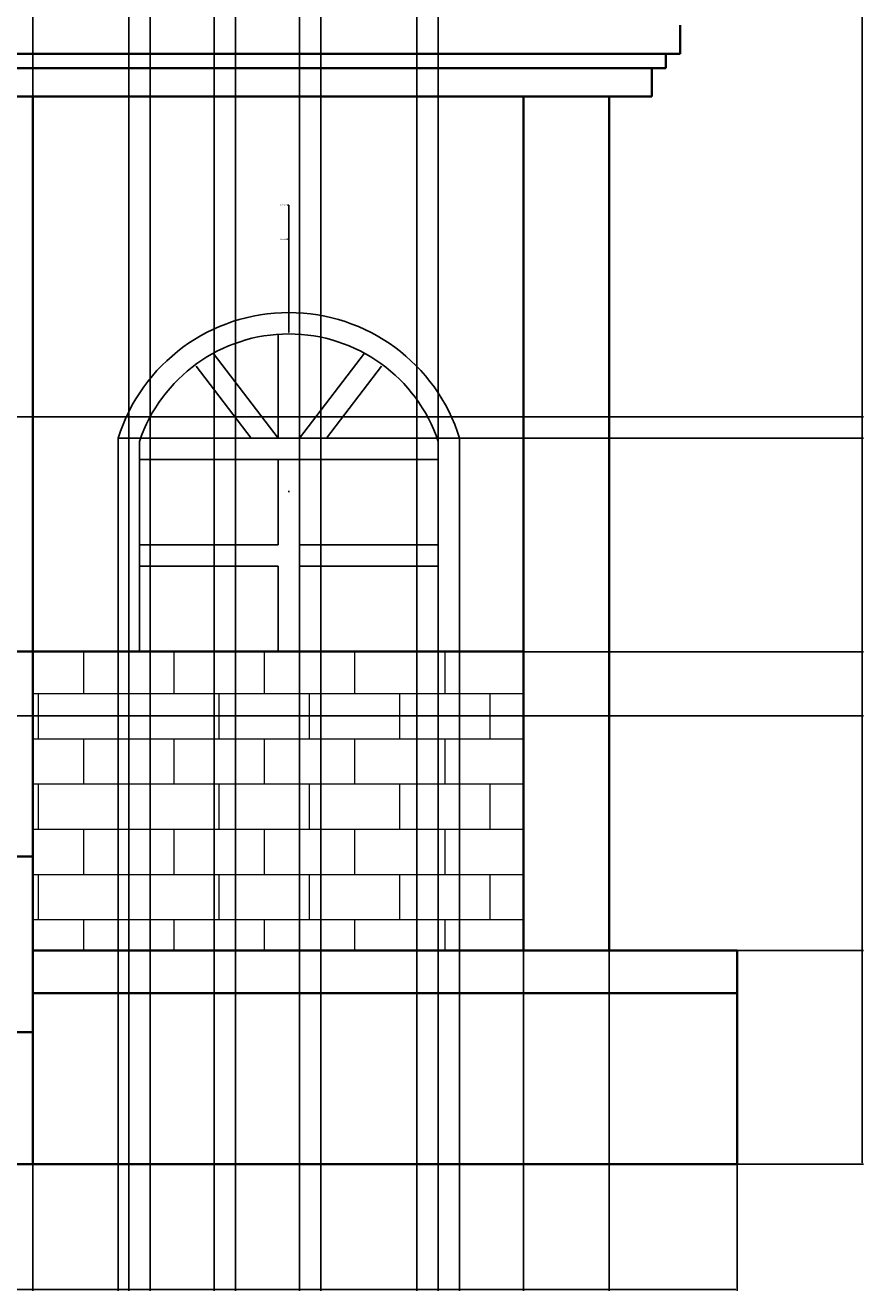
# Model space of a CAD drawing. Units: inches. Extents: x 2612 to 2948, y 481 to 865.
# Tile 4 of 7: x 2830 to 2948, y 481 to 659. Entities that reach past the tile are written whole.
import ezdxf

# ---------------------------------------------------------------- set-up
doc = ezdxf.new("R2010")
doc.units = ezdxf.units.IN
for name, color, linetype, lineweight in [('A-ANNO-DIMS', 2, 'Continuous', 18), ('A-COLS', 1, 'Continuous', 35), ('A-ELEV', 7, 'Continuous', 35), ('A-GLAZ', 4, 'Continuous', 25), ('A-WALL-PATT', 8, 'Continuous', 13)]:
    doc.layers.add(name, color=color, linetype=linetype, lineweight=lineweight)
doc.styles.get("Standard").update_dxf_attribs({"font": 'arial.ttf'})
doc.dimstyles.get("Standard").update_dxf_attribs({"dimtxt": 0.18, "dimasz": 0.18, "dimexe": 0.18, "dimexo": 0.0625, "dimgap": 0.09, "dimtad": 0, "dimtih": 1, "dimtoh": 1, "dimdec": 4, "dimzin": 0, "dimdsep": 46, "dimtxsty": 'Standard', "dimcen": 0.09, "dimadec": 0, "dimazin": 0, "dimtfac": 1, "dimtdec": 4, "dimtofl": 0, "dimtmove": 0, "dimatfit": 3, "dimfxl": 1, "dimtolj": 1, "dimtzin": 0, "dimarcsym": 0})

# ---------------------------------------------------------------- blocks, each defined once
blk = doc.blocks.new('*D12')
at = {"layer": 'A-ANNO-DIMS', "color": 0, "lineweight": -2, "transparency": 16777216}
for p, q in [((2930.37, 529.04), (2948.09, 529.04)), ((2947.91, 528.86), (2947.91, 514.23)), ((2947.91, 499.22), (2947.91, 513.86)), ((2930.37, 499.04), (2948.09, 499.04))]:
    blk.add_line(p, q, dxfattribs=at)
at = {"layer": 'A-ANNO-DIMS', "color": 0, "transparency": 16777216}
for points in [[(2947.88, 528.86), (2947.94, 528.86), (2947.91, 529.04)], [(2947.88, 499.22), (2947.94, 499.22), (2947.91, 499.04)]]:
    blk.add_solid(points, dxfattribs=at)
at = {"layer": 'Defpoints', "color": 0, "transparency": 16777216}
for p in [(2930.31, 529.04), (2947.91, 529.04), (2930.31, 499.04)]:
    blk.add_point(p, dxfattribs=at)
at = {"layer": 'A-ANNO-DIMS', "color": 0, "transparency": 16777216, "insert": (2947.91, 514.04), "char_height": 0.18, "attachment_point": 5}
blk.add_mtext('\\A1;30', dxfattribs=at)
blk = doc.blocks.new('*D13')
at = {"layer": 'A-ANNO-DIMS', "color": 0, "lineweight": -2, "transparency": 16777216}
for p, q in [((2843.37, 571.04), (2948.09, 571.04)), ((2947.91, 570.86), (2947.91, 550.22)), ((2947.91, 529.22), (2947.91, 549.86)), ((2930.37, 529.04), (2948.09, 529.04))]:
    blk.add_line(p, q, dxfattribs=at)
at = {"layer": 'A-ANNO-DIMS', "color": 0, "transparency": 16777216}
for points in [[(2947.88, 570.86), (2947.94, 570.86), (2947.91, 571.04)], [(2947.88, 529.22), (2947.94, 529.22), (2947.91, 529.04)]]:
    blk.add_solid(points, dxfattribs=at)
at = {"layer": 'Defpoints', "color": 0, "transparency": 16777216}
for p in [(2843.31, 571.04), (2947.91, 571.04), (2930.31, 529.04)]:
    blk.add_point(p, dxfattribs=at)
at = {"layer": 'A-ANNO-DIMS', "color": 0, "transparency": 16777216, "insert": (2947.91, 550.04), "char_height": 0.18, "attachment_point": 5}
blk.add_mtext('\\A1;42', dxfattribs=at)
blk = doc.blocks.new('*D14')
at = {"layer": 'A-ANNO-DIMS', "color": 0, "lineweight": -2, "transparency": 16777216}
for p, q in [((2843.37, 601.04), (2948.09, 601.04)), ((2947.91, 600.86), (2947.91, 586.23)), ((2947.91, 571.22), (2947.91, 585.86)), ((2843.37, 571.04), (2948.09, 571.04))]:
    blk.add_line(p, q, dxfattribs=at)
at = {"layer": 'A-ANNO-DIMS', "color": 0, "transparency": 16777216}
for points in [[(2947.88, 600.86), (2947.94, 600.86), (2947.91, 601.04)], [(2947.88, 571.22), (2947.94, 571.22), (2947.91, 571.04)]]:
    blk.add_solid(points, dxfattribs=at)
at = {"layer": 'Defpoints', "color": 0, "transparency": 16777216}
for p in [(2843.31, 601.04), (2947.91, 601.04), (2843.31, 571.04)]:
    blk.add_point(p, dxfattribs=at)
at = {"layer": 'A-ANNO-DIMS', "color": 0, "transparency": 16777216, "insert": (2947.91, 586.04), "char_height": 0.18, "attachment_point": 5}
blk.add_mtext('\\A1;30', dxfattribs=at)
blk = doc.blocks.new('*D22')
at = {"layer": 'A-ANNO-DIMS', "color": 0, "lineweight": -2, "transparency": 16777216}
for p, q in [((2708.31, 648.98), (2708.31, 481.26)), ((2831.31, 570.98), (2831.31, 481.26)), ((2708.49, 481.44), (2769.53, 481.44)), ((2831.13, 481.44), (2770.09, 481.44))]:
    blk.add_line(p, q, dxfattribs=at)
at = {"layer": 'A-ANNO-DIMS', "color": 0, "transparency": 16777216}
for points in [[(2708.49, 481.47), (2708.49, 481.41), (2708.31, 481.44)], [(2831.13, 481.47), (2831.13, 481.41), (2831.31, 481.44)]]:
    blk.add_solid(points, dxfattribs=at)
at = {"layer": 'Defpoints', "color": 0, "transparency": 16777216}
for p in [(2708.31, 649.04), (2831.31, 571.04), (2831.31, 481.44)]:
    blk.add_point(p, dxfattribs=at)
at = {"layer": 'A-ANNO-DIMS', "color": 0, "transparency": 16777216, "insert": (2769.81, 481.44), "char_height": 0.18, "attachment_point": 5}
blk.add_mtext('\\A1;123', dxfattribs=at)
blk = doc.blocks.new('*D23')
at = {"layer": 'A-ANNO-DIMS', "color": 0, "lineweight": -2, "transparency": 16777216}
for p, q in [((2831.31, 570.98), (2831.31, 481.26)), ((2843.31, 570.98), (2843.31, 481.26)), ((2831.49, 481.44), (2837.1, 481.44)), ((2843.13, 481.44), (2837.52, 481.44))]:
    blk.add_line(p, q, dxfattribs=at)
at = {"layer": 'A-ANNO-DIMS', "color": 0, "transparency": 16777216}
for points in [[(2831.49, 481.47), (2831.49, 481.41), (2831.31, 481.44)], [(2843.13, 481.47), (2843.13, 481.41), (2843.31, 481.44)]]:
    blk.add_solid(points, dxfattribs=at)
at = {"layer": 'Defpoints', "color": 0, "transparency": 16777216}
for p in [(2831.31, 571.04), (2843.31, 571.04), (2843.31, 481.44)]:
    blk.add_point(p, dxfattribs=at)
at = {"layer": 'A-ANNO-DIMS', "color": 0, "transparency": 16777216, "insert": (2837.31, 481.44), "char_height": 0.18, "attachment_point": 5}
blk.add_mtext('\\A1;12', dxfattribs=at)
blk = doc.blocks.new('*D24')
at = {"layer": 'A-ANNO-DIMS', "color": 0, "lineweight": -2, "transparency": 16777216}
for p, q in [((2843.31, 570.98), (2843.31, 481.26)), ((2891.31, 570.98), (2891.31, 481.26)), ((2843.49, 481.44), (2867.08, 481.44)), ((2891.13, 481.44), (2867.53, 481.44))]:
    blk.add_line(p, q, dxfattribs=at)
at = {"layer": 'A-ANNO-DIMS', "color": 0, "transparency": 16777216}
for points in [[(2843.49, 481.47), (2843.49, 481.41), (2843.31, 481.44)], [(2891.13, 481.47), (2891.13, 481.41), (2891.31, 481.44)]]:
    blk.add_solid(points, dxfattribs=at)
at = {"layer": 'Defpoints', "color": 0, "transparency": 16777216}
for p in [(2843.31, 571.04), (2891.31, 571.04), (2891.31, 481.44)]:
    blk.add_point(p, dxfattribs=at)
at = {"layer": 'A-ANNO-DIMS', "color": 0, "transparency": 16777216, "insert": (2867.31, 481.44), "char_height": 0.18, "attachment_point": 5}
blk.add_mtext('\\A1;48', dxfattribs=at)
blk = doc.blocks.new('*D25')
at = {"layer": 'A-ANNO-DIMS', "color": 0, "lineweight": -2, "transparency": 16777216}
for p, q in [((2891.31, 570.98), (2891.31, 481.26)), ((2900.31, 570.98), (2900.31, 481.26)), ((2891.49, 481.44), (2895.66, 481.44)), ((2900.13, 481.44), (2895.96, 481.44))]:
    blk.add_line(p, q, dxfattribs=at)
at = {"layer": 'A-ANNO-DIMS', "color": 0, "transparency": 16777216}
for points in [[(2891.49, 481.47), (2891.49, 481.41), (2891.31, 481.44)], [(2900.13, 481.47), (2900.13, 481.41), (2900.31, 481.44)]]:
    blk.add_solid(points, dxfattribs=at)
at = {"layer": 'Defpoints', "color": 0, "transparency": 16777216}
for p in [(2891.31, 571.04), (2900.31, 571.04), (2900.31, 481.44)]:
    blk.add_point(p, dxfattribs=at)
at = {"layer": 'A-ANNO-DIMS', "color": 0, "transparency": 16777216, "insert": (2895.81, 481.44), "char_height": 0.18, "attachment_point": 5}
blk.add_mtext('\\A1;9', dxfattribs=at)
blk = doc.blocks.new('*D26')
at = {"layer": 'A-ANNO-DIMS', "color": 0, "lineweight": -2, "transparency": 16777216}
for p, q in [((2900.31, 528.98), (2900.31, 481.26)), ((2912.31, 528.98), (2912.31, 481.26)), ((2900.49, 481.44), (2906.1, 481.44)), ((2912.13, 481.44), (2906.52, 481.44))]:
    blk.add_line(p, q, dxfattribs=at)
at = {"layer": 'A-ANNO-DIMS', "color": 0, "transparency": 16777216}
for points in [[(2900.49, 481.47), (2900.49, 481.41), (2900.31, 481.44)], [(2912.13, 481.47), (2912.13, 481.41), (2912.31, 481.44)]]:
    blk.add_solid(points, dxfattribs=at)
at = {"layer": 'Defpoints', "color": 0, "transparency": 16777216}
for p in [(2900.31, 529.04), (2912.31, 529.04), (2912.31, 481.44)]:
    blk.add_point(p, dxfattribs=at)
at = {"layer": 'A-ANNO-DIMS', "color": 0, "transparency": 16777216, "insert": (2906.31, 481.44), "char_height": 0.18, "attachment_point": 5}
blk.add_mtext('\\A1;12', dxfattribs=at)
blk = doc.blocks.new('*D27')
at = {"layer": 'A-ANNO-DIMS', "color": 0, "lineweight": -2, "transparency": 16777216}
for p, q in [((2912.31, 528.98), (2912.31, 481.26)), ((2930.31, 528.98), (2930.31, 481.26)), ((2912.49, 481.44), (2921.1, 481.44)), ((2930.13, 481.44), (2921.52, 481.44))]:
    blk.add_line(p, q, dxfattribs=at)
at = {"layer": 'A-ANNO-DIMS', "color": 0, "transparency": 16777216}
for points in [[(2912.49, 481.47), (2912.49, 481.41), (2912.31, 481.44)], [(2930.13, 481.47), (2930.13, 481.41), (2930.31, 481.44)]]:
    blk.add_solid(points, dxfattribs=at)
at = {"layer": 'Defpoints', "color": 0, "transparency": 16777216}
for p in [(2912.31, 529.04), (2930.31, 529.04), (2930.31, 481.44)]:
    blk.add_point(p, dxfattribs=at)
at = {"layer": 'A-ANNO-DIMS', "color": 0, "transparency": 16777216, "insert": (2921.31, 481.44), "char_height": 0.18, "attachment_point": 5}
blk.add_mtext('\\A1;18', dxfattribs=at)
blk = doc.blocks.new('*D64')
at = {"layer": 'A-ANNO-DIMS', "color": 0, "lineweight": -2, "transparency": 16777216}
for p, q in [((2826.87, 562.04), (2948.09, 562.04)), ((2947.91, 561.86), (2947.91, 530.73)), ((2947.91, 499.22), (2947.91, 530.36)), ((2826.87, 499.04), (2948.09, 499.04))]:
    blk.add_line(p, q, dxfattribs=at)
at = {"layer": 'A-ANNO-DIMS', "color": 0, "transparency": 16777216}
for points in [[(2947.88, 561.86), (2947.94, 561.86), (2947.91, 562.04)], [(2947.88, 499.22), (2947.94, 499.22), (2947.91, 499.04)]]:
    blk.add_solid(points, dxfattribs=at)
at = {"layer": 'Defpoints', "color": 0, "transparency": 16777216}
for p in [(2826.81, 562.04), (2947.91, 562.04), (2826.81, 499.04)]:
    blk.add_point(p, dxfattribs=at)
at = {"layer": 'A-ANNO-DIMS', "color": 0, "transparency": 16777216, "insert": (2947.91, 530.54), "char_height": 0.18, "attachment_point": 5}
blk.add_mtext('\\A1;63', dxfattribs=at)
blk = doc.blocks.new('*D65')
at = {"layer": 'A-ANNO-DIMS', "color": 0, "lineweight": -2, "transparency": 16777216}
for p, q in [((2793.87, 604.04), (2948.09, 604.04)), ((2947.91, 603.86), (2947.91, 583.22)), ((2947.91, 562.22), (2947.91, 582.86)), ((2793.87, 562.04), (2948.09, 562.04))]:
    blk.add_line(p, q, dxfattribs=at)
at = {"layer": 'A-ANNO-DIMS', "color": 0, "transparency": 16777216}
for points in [[(2947.88, 603.86), (2947.94, 603.86), (2947.91, 604.04)], [(2947.88, 562.22), (2947.94, 562.22), (2947.91, 562.04)]]:
    blk.add_solid(points, dxfattribs=at)
at = {"layer": 'Defpoints', "color": 0, "transparency": 16777216}
for p in [(2793.81, 604.04), (2947.91, 604.04), (2793.81, 562.04)]:
    blk.add_point(p, dxfattribs=at)
at = {"layer": 'A-ANNO-DIMS', "color": 0, "transparency": 16777216, "insert": (2947.91, 583.04), "char_height": 0.18, "attachment_point": 5}
blk.add_mtext('\\A1;42', dxfattribs=at)
blk = doc.blocks.new('*D74')
at = {"layer": 'A-ANNO-DIMS', "color": 0, "lineweight": -2, "transparency": 16777216}
for p, q in [((2831.31, 711.98), (2831.31, 481.26)), ((2828.31, 708.98), (2828.31, 481.26)), ((2828.49, 481.44), (2829.66, 481.44)), ((2831.13, 481.44), (2829.96, 481.44))]:
    blk.add_line(p, q, dxfattribs=at)
at = {"layer": 'A-ANNO-DIMS', "color": 0, "transparency": 16777216}
for points in [[(2828.49, 481.47), (2828.49, 481.41), (2828.31, 481.44)], [(2831.13, 481.47), (2831.13, 481.41), (2831.31, 481.44)]]:
    blk.add_solid(points, dxfattribs=at)
at = {"layer": 'Defpoints', "color": 0, "transparency": 16777216}
for p in [(2831.31, 712.04), (2828.31, 709.04), (2831.31, 481.44)]:
    blk.add_point(p, dxfattribs=at)
at = {"layer": 'A-ANNO-DIMS', "color": 0, "transparency": 16777216, "insert": (2829.81, 481.44), "char_height": 0.18, "attachment_point": 5}
blk.add_mtext('\\A1;3', dxfattribs=at)
blk = doc.blocks.new('*D75')
at = {"layer": 'A-ANNO-DIMS', "color": 0, "lineweight": -2, "transparency": 16777216}
for p, q in [((2831.31, 711.98), (2831.31, 481.26)), ((2844.81, 711.98), (2844.81, 481.26)), ((2831.49, 481.44), (2837.74, 481.44)), ((2844.63, 481.44), (2838.37, 481.44))]:
    blk.add_line(p, q, dxfattribs=at)
at = {"layer": 'A-ANNO-DIMS', "color": 0, "transparency": 16777216}
for points in [[(2831.49, 481.47), (2831.49, 481.41), (2831.31, 481.44)], [(2844.63, 481.47), (2844.63, 481.41), (2844.81, 481.44)]]:
    blk.add_solid(points, dxfattribs=at)
at = {"layer": 'Defpoints', "color": 0, "transparency": 16777216}
for p in [(2831.31, 712.04), (2844.81, 712.04), (2844.81, 481.44)]:
    blk.add_point(p, dxfattribs=at)
at = {"layer": 'A-ANNO-DIMS', "color": 0, "transparency": 16777216, "insert": (2838.06, 481.44), "char_height": 0.18, "attachment_point": 5}
blk.add_mtext('\\A1;13.5', dxfattribs=at)
blk = doc.blocks.new('*D76')
at = {"layer": 'A-ANNO-DIMS', "color": 0, "lineweight": -2, "transparency": 16777216}
for p, q in [((2844.81, 711.98), (2844.81, 481.26)), ((2847.81, 711.98), (2847.81, 481.26)), ((2844.99, 481.44), (2846.16, 481.44)), ((2847.63, 481.44), (2846.46, 481.44))]:
    blk.add_line(p, q, dxfattribs=at)
at = {"layer": 'A-ANNO-DIMS', "color": 0, "transparency": 16777216}
for points in [[(2844.99, 481.47), (2844.99, 481.41), (2844.81, 481.44)], [(2847.63, 481.47), (2847.63, 481.41), (2847.81, 481.44)]]:
    blk.add_solid(points, dxfattribs=at)
at = {"layer": 'Defpoints', "color": 0, "transparency": 16777216}
for p in [(2844.81, 712.04), (2847.81, 712.04), (2847.81, 481.44)]:
    blk.add_point(p, dxfattribs=at)
at = {"layer": 'A-ANNO-DIMS', "color": 0, "transparency": 16777216, "insert": (2846.31, 481.44), "char_height": 0.18, "attachment_point": 5}
blk.add_mtext('\\A1;3', dxfattribs=at)
blk = doc.blocks.new('*D77')
at = {"layer": 'A-ANNO-DIMS', "color": 0, "lineweight": -2, "transparency": 16777216}
for p, q in [((2847.81, 711.98), (2847.81, 481.26)), ((2856.81, 711.98), (2856.81, 481.26)), ((2847.99, 481.44), (2852.16, 481.44)), ((2856.63, 481.44), (2852.46, 481.44))]:
    blk.add_line(p, q, dxfattribs=at)
at = {"layer": 'A-ANNO-DIMS', "color": 0, "transparency": 16777216}
for points in [[(2847.99, 481.47), (2847.99, 481.41), (2847.81, 481.44)], [(2856.63, 481.47), (2856.63, 481.41), (2856.81, 481.44)]]:
    blk.add_solid(points, dxfattribs=at)
at = {"layer": 'Defpoints', "color": 0, "transparency": 16777216}
for p in [(2847.81, 712.04), (2856.81, 712.04), (2856.81, 481.44)]:
    blk.add_point(p, dxfattribs=at)
at = {"layer": 'A-ANNO-DIMS', "color": 0, "transparency": 16777216, "insert": (2852.31, 481.44), "char_height": 0.18, "attachment_point": 5}
blk.add_mtext('\\A1;9', dxfattribs=at)
blk = doc.blocks.new('*D78')
at = {"layer": 'A-ANNO-DIMS', "color": 0, "lineweight": -2, "transparency": 16777216}
for p, q in [((2856.81, 711.98), (2856.81, 481.26)), ((2859.81, 711.98), (2859.81, 481.26)), ((2856.99, 481.44), (2858.16, 481.44)), ((2859.63, 481.44), (2858.46, 481.44))]:
    blk.add_line(p, q, dxfattribs=at)
at = {"layer": 'A-ANNO-DIMS', "color": 0, "transparency": 16777216}
for points in [[(2856.99, 481.47), (2856.99, 481.41), (2856.81, 481.44)], [(2859.63, 481.47), (2859.63, 481.41), (2859.81, 481.44)]]:
    blk.add_solid(points, dxfattribs=at)
at = {"layer": 'Defpoints', "color": 0, "transparency": 16777216}
for p in [(2856.81, 712.04), (2859.81, 712.04), (2859.81, 481.44)]:
    blk.add_point(p, dxfattribs=at)
at = {"layer": 'A-ANNO-DIMS', "color": 0, "transparency": 16777216, "insert": (2858.31, 481.44), "char_height": 0.18, "attachment_point": 5}
blk.add_mtext('\\A1;3', dxfattribs=at)
blk = doc.blocks.new('*D79')
at = {"layer": 'A-ANNO-DIMS', "color": 0, "lineweight": -2, "transparency": 16777216}
for p, q in [((2859.81, 711.98), (2859.81, 481.26)), ((2868.81, 711.98), (2868.81, 481.26)), ((2859.99, 481.44), (2864.16, 481.44)), ((2868.63, 481.44), (2864.46, 481.44))]:
    blk.add_line(p, q, dxfattribs=at)
at = {"layer": 'A-ANNO-DIMS', "color": 0, "transparency": 16777216}
for points in [[(2859.99, 481.47), (2859.99, 481.41), (2859.81, 481.44)], [(2868.63, 481.47), (2868.63, 481.41), (2868.81, 481.44)]]:
    blk.add_solid(points, dxfattribs=at)
at = {"layer": 'Defpoints', "color": 0, "transparency": 16777216}
for p in [(2859.81, 712.04), (2868.81, 712.04), (2868.81, 481.44)]:
    blk.add_point(p, dxfattribs=at)
at = {"layer": 'A-ANNO-DIMS', "color": 0, "transparency": 16777216, "insert": (2864.31, 481.44), "char_height": 0.18, "attachment_point": 5}
blk.add_mtext('\\A1;9', dxfattribs=at)
blk = doc.blocks.new('*D80')
at = {"layer": 'A-ANNO-DIMS', "color": 0, "lineweight": -2, "transparency": 16777216}
for p, q in [((2868.81, 711.98), (2868.81, 481.26)), ((2871.81, 711.98), (2871.81, 481.26)), ((2868.99, 481.44), (2870.16, 481.44)), ((2871.63, 481.44), (2870.46, 481.44))]:
    blk.add_line(p, q, dxfattribs=at)
at = {"layer": 'A-ANNO-DIMS', "color": 0, "transparency": 16777216}
for points in [[(2868.99, 481.47), (2868.99, 481.41), (2868.81, 481.44)], [(2871.63, 481.47), (2871.63, 481.41), (2871.81, 481.44)]]:
    blk.add_solid(points, dxfattribs=at)
at = {"layer": 'Defpoints', "color": 0, "transparency": 16777216}
for p in [(2868.81, 712.04), (2871.81, 712.04), (2871.81, 481.44)]:
    blk.add_point(p, dxfattribs=at)
at = {"layer": 'A-ANNO-DIMS', "color": 0, "transparency": 16777216, "insert": (2870.31, 481.44), "char_height": 0.18, "attachment_point": 5}
blk.add_mtext('\\A1;3', dxfattribs=at)
blk = doc.blocks.new('*D81')
at = {"layer": 'A-ANNO-DIMS', "color": 0, "lineweight": -2, "transparency": 16777216}
for p, q in [((2871.81, 711.98), (2871.81, 481.26)), ((2885.31, 711.98), (2885.31, 481.26)), ((2871.99, 481.44), (2878.24, 481.44)), ((2885.13, 481.44), (2878.87, 481.44))]:
    blk.add_line(p, q, dxfattribs=at)
at = {"layer": 'A-ANNO-DIMS', "color": 0, "transparency": 16777216}
for points in [[(2871.99, 481.47), (2871.99, 481.41), (2871.81, 481.44)], [(2885.13, 481.47), (2885.13, 481.41), (2885.31, 481.44)]]:
    blk.add_solid(points, dxfattribs=at)
at = {"layer": 'Defpoints', "color": 0, "transparency": 16777216}
for p in [(2871.81, 712.04), (2885.31, 712.04), (2885.31, 481.44)]:
    blk.add_point(p, dxfattribs=at)
at = {"layer": 'A-ANNO-DIMS', "color": 0, "transparency": 16777216, "insert": (2878.56, 481.44), "char_height": 0.18, "attachment_point": 5}
blk.add_mtext('\\A1;13.5', dxfattribs=at)
blk = doc.blocks.new('*D82')
at = {"layer": 'A-ANNO-DIMS', "color": 0, "lineweight": -2, "transparency": 16777216}
for p, q in [((2885.31, 711.98), (2885.31, 481.26)), ((2888.31, 708.98), (2888.31, 481.26)), ((2885.49, 481.44), (2886.66, 481.44)), ((2888.13, 481.44), (2886.96, 481.44))]:
    blk.add_line(p, q, dxfattribs=at)
at = {"layer": 'A-ANNO-DIMS', "color": 0, "transparency": 16777216}
for points in [[(2885.49, 481.47), (2885.49, 481.41), (2885.31, 481.44)], [(2888.13, 481.47), (2888.13, 481.41), (2888.31, 481.44)]]:
    blk.add_solid(points, dxfattribs=at)
at = {"layer": 'Defpoints', "color": 0, "transparency": 16777216}
for p in [(2885.31, 712.04), (2888.31, 709.04), (2888.31, 481.44)]:
    blk.add_point(p, dxfattribs=at)
at = {"layer": 'A-ANNO-DIMS', "color": 0, "transparency": 16777216, "insert": (2886.81, 481.44), "char_height": 0.18, "attachment_point": 5}
blk.add_mtext('\\A1;3', dxfattribs=at)
blk = doc.blocks.new('*D86')
at = {"layer": 'A-ANNO-DIMS', "color": 0, "lineweight": -2, "transparency": 16777216}
for p, q in [((2930.37, 847.04), (2948.09, 847.04)), ((2947.91, 846.86), (2947.91, 673.23)), ((2947.91, 499.22), (2947.91, 672.86)), ((2930.37, 499.04), (2948.09, 499.04))]:
    blk.add_line(p, q, dxfattribs=at)
at = {"layer": 'A-ANNO-DIMS', "color": 0, "transparency": 16777216}
for points in [[(2947.88, 846.86), (2947.94, 846.86), (2947.91, 847.04)], [(2947.88, 499.22), (2947.94, 499.22), (2947.91, 499.04)]]:
    blk.add_solid(points, dxfattribs=at)
at = {"layer": 'Defpoints', "color": 0, "transparency": 16777216}
for p in [(2930.31, 847.04), (2947.91, 847.04), (2930.31, 499.04)]:
    blk.add_point(p, dxfattribs=at)
at = {"layer": 'A-ANNO-DIMS', "color": 0, "transparency": 16777216, "insert": (2947.91, 673.04), "char_height": 0.18, "attachment_point": 5}
blk.add_mtext('\\A1;348', dxfattribs=at)
blk = doc.blocks.new('*D87')
at = {"layer": 'A-ANNO-DIMS', "color": 0, "lineweight": -2, "transparency": 16777216}
for p, q in [((2630.31, 498.98), (2630.31, 481.26)), ((2930.31, 498.98), (2930.31, 481.26)), ((2630.49, 481.44), (2780.02, 481.44)), ((2930.13, 481.44), (2780.6, 481.44))]:
    blk.add_line(p, q, dxfattribs=at)
at = {"layer": 'A-ANNO-DIMS', "color": 0, "transparency": 16777216}
for points in [[(2630.49, 481.47), (2630.49, 481.41), (2630.31, 481.44)], [(2930.13, 481.47), (2930.13, 481.41), (2930.31, 481.44)]]:
    blk.add_solid(points, dxfattribs=at)
at = {"layer": 'Defpoints', "color": 0, "transparency": 16777216}
for p in [(2630.31, 499.04), (2930.31, 499.04), (2930.31, 481.44)]:
    blk.add_point(p, dxfattribs=at)
at = {"layer": 'A-ANNO-DIMS', "color": 0, "transparency": 16777216, "insert": (2780.31, 481.44), "char_height": 0.18, "attachment_point": 5}
blk.add_mtext('\\A1;300', dxfattribs=at)
blk = doc.blocks.new('*D88')
at = {"layer": 'A-ANNO-DIMS', "color": 0, "lineweight": -2, "transparency": 16777216}
for p, q in [((2867.13, 633.78), (2867.31, 633.78)), ((2867.31, 633.78), (2867.31, 618.87)), ((2867.22, 593.54), (2867.4, 593.54)), ((2867.31, 593.45), (2867.31, 593.63))]:
    blk.add_line(p, q, dxfattribs=at)
at = {"layer": 'A-ANNO-DIMS', "color": 0, "transparency": 16777216}
blk.add_solid([(2867.34, 618.87), (2867.28, 618.87), (2867.31, 618.69)], dxfattribs=at)
at = {"layer": 'Defpoints', "color": 0, "transparency": 16777216}
for p in [(2867.31, 618.69), (2867.31, 593.54)]:
    blk.add_point(p, dxfattribs=at)
at = {"layer": 'A-ANNO-DIMS', "color": 0, "transparency": 16777216, "insert": (2866.58, 633.78), "char_height": 0.18, "attachment_point": 5}
blk.add_mtext('\\A1;R25.145', dxfattribs=at)
blk = doc.blocks.new('*D89')
at = {"layer": 'A-ANNO-DIMS', "color": 0, "lineweight": -2, "transparency": 16777216}
for p, q in [((2867.13, 628.98), (2867.31, 628.98)), ((2867.31, 628.98), (2867.31, 615.87)), ((2867.22, 593.54), (2867.4, 593.54)), ((2867.31, 593.45), (2867.31, 593.63))]:
    blk.add_line(p, q, dxfattribs=at)
at = {"layer": 'A-ANNO-DIMS', "color": 0, "transparency": 16777216}
blk.add_solid([(2867.34, 615.87), (2867.28, 615.87), (2867.31, 615.69)], dxfattribs=at)
at = {"layer": 'Defpoints', "color": 0, "transparency": 16777216}
for p in [(2867.31, 615.69), (2867.31, 593.54)]:
    blk.add_point(p, dxfattribs=at)
at = {"layer": 'A-ANNO-DIMS', "color": 0, "transparency": 16777216, "insert": (2866.58, 628.98), "char_height": 0.18, "attachment_point": 5}
blk.add_mtext('\\A1;R22.145', dxfattribs=at)

msp = doc.modelspace()

# ---------------------------------------------------------------- hatches: boundary and pattern name
at = {"layer": 'A-WALL-PATT'}
h = msp.add_hatch(dxfattribs=at)
h.set_pattern_fill('BRICK', color=256)
h.paths.add_polyline_path([(2900.3074, 571.0443), (2831.3074, 571.0443), (2831.3074, 529.0443), (2900.3074, 529.0443)])

# ---------------------------------------------------------------- linework, layer by layer
at = {"layer": 'A-COLS'}
msp.add_line((2900.3074, 529.0443), (2900.3074, 649.0443), dxfattribs=at)
at = {"layer": 'A-ELEV'}
for p, q in [((2922.3074, 655.0443), (2922.3074, 659.0443)), ((2642.3074, 655.0443), (2918.3074, 655.0443)), ((2918.3074, 655.0443), (2920.3074, 655.0443)), ((2920.3074, 655.0443), (2922.3074, 655.0443)), ((2920.3074, 653.0443), (2920.3074, 655.0443)), ((2642.3074, 653.0443), (2918.3074, 653.0443)), ((2918.3074, 649.0443), (2918.3074, 653.0443)), ((2918.3074, 653.0443), (2920.3074, 653.0443)), ((2642.3074, 649.0443), (2918.3074, 649.0443)), ((2831.3074, 499.0443), (2831.3074, 649.0443)), ((2912.3074, 529.0443), (2912.3074, 649.0443)), ((2816.9214, 571.0443), (2900.3074, 571.0443)), ((2831.3074, 571.0443), (2816.9214, 571.0443)), ((2826.8074, 542.2613), (2831.3074, 542.2613)), ((2831.3074, 529.0443), (2900.3074, 529.0443)), ((2900.3074, 529.0443), (2930.3074, 529.0443)), ((2930.3074, 499.0443), (2930.3074, 529.0443)), ((2831.3074, 523.0443), (2900.3074, 523.0443)), ((2900.3074, 523.0443), (2930.3074, 523.0443)), ((2826.8074, 517.5686), (2831.3074, 517.5686)), ((2630.3074, 499.0443), (2930.3074, 499.0443))]:
    msp.add_line(p, q, dxfattribs=at)
at = {"layer": 'A-GLAZ'}
for p, q in [((2865.8074, 601.0443), (2865.8074, 615.6889)), ((2868.8074, 601.0443), (2868.8074, 615.6889)), ((2865.8074, 601.0443), (2856.6574, 612.9597)), ((2868.8074, 601.0443), (2877.9575, 612.9597)), ((2862.0249, 601.0443), (2854.278, 611.1326)), ((2872.5899, 601.0443), (2880.3368, 611.1326)), ((2843.3074, 571.0443), (2843.3074, 601.0443)), ((2846.4716, 601.0443), (2862.0249, 601.0443)), ((2872.5899, 601.0443), (2888.1433, 601.0443)), ((2891.3074, 571.0443), (2891.3074, 601.0443)), ((2846.3074, 571.0443), (2846.3074, 600.5715)), ((2888.3074, 571.0443), (2888.3074, 600.5715)), ((2846.3074, 598.0443), (2865.8074, 598.0443)), ((2865.8074, 598.0443), (2865.8074, 586.0443)), ((2865.8074, 598.0443), (2888.3074, 598.0443)), ((2868.8074, 598.0443), (2868.8074, 586.0443)), ((2846.3074, 586.0443), (2865.8074, 586.0443)), ((2868.8074, 586.0443), (2888.3074, 586.0443)), ((2846.3074, 583.0443), (2865.8074, 583.0443)), ((2865.8074, 583.0443), (2865.8074, 571.0443)), ((2865.8074, 583.0443), (2865.8074, 571.0443)), ((2868.8074, 583.0443), (2868.8074, 571.0443)), ((2868.8074, 583.0443), (2888.3074, 583.0443)), ((2868.8074, 583.0443), (2868.8074, 571.0443)), ((2843.3074, 571.0443), (2891.3074, 571.0443))]:
    msp.add_line(p, q, dxfattribs=at)
for radius, start, end in [(25.1446, 17.354025, 162.645975), (22.1446, 18.501882, 161.498118)]:
    msp.add_arc((2867.3074, 593.5443), radius, start, end, dxfattribs=at)

# ---------------------------------------------------------------- dimensions: what is measured, and where the dimension line sits
at = {"layer": 'A-ANNO-DIMS'}
for base, p1, p2, picture, middle in [((2947.9074, 847.0443), (2930.3074, 499.0443), (2930.3074, 847.0443), '*D86', (2947.9074, 673.0443)), ((2947.9074, 604.0443), (2793.8074, 562.0443), (2793.8074, 604.0443), '*D65', (2947.9074, 583.0443)), ((2947.9074, 601.0443), (2843.3074, 571.0443), (2843.3074, 601.0443), '*D14', (2947.9074, 586.0443)), ((2947.9074, 571.0443), (2930.3074, 529.0443), (2843.3074, 571.0443), '*D13', (2947.9074, 550.0443)), ((2947.9074, 562.0443), (2826.8074, 499.0443), (2826.8074, 562.0443), '*D64', (2947.9074, 530.5443)), ((2947.9074, 529.0443), (2930.3074, 499.0443), (2930.3074, 529.0443), '*D12', (2947.9074, 514.0443))]:
    dim = msp.add_linear_dim(base=base, p1=p1, p2=p2, angle=90, dimstyle='Standard', override={"dimdec": 0, "dimlfac": 1, "dimrnd": 0, "dimzin": 0, "dimdsep": 46, "dimlunit": 2}, dxfattribs=at)
    dim.commit()
    dim.dimension.update_dxf_attribs({"geometry": picture, "text_midpoint": middle})
for base, p1, p2, override, picture, middle in [((2831.3074, 481.4443), (2828.3074, 709.0443), (2831.3074, 712.0443), {"dimdec": 0, "dimlfac": 1, "dimrnd": 0, "dimzin": 0, "dimdsep": 46, "dimlunit": 2}, '*D74', (2829.8074, 481.4443)), ((2844.8074, 481.4443), (2831.3074, 712.0443), (2844.8074, 712.0443), {"dimdec": 1, "dimlfac": 1, "dimrnd": 0, "dimzin": 0, "dimdsep": 46, "dimlunit": 2}, '*D75', (2838.0574, 481.4443)), ((2847.8074, 481.4443), (2844.8074, 712.0443), (2847.8074, 712.0443), {"dimdec": 0, "dimlfac": 1, "dimrnd": 0, "dimzin": 0, "dimdsep": 46, "dimlunit": 2}, '*D76', (2846.3074, 481.4443)), ((2856.8074, 481.4443), (2847.8074, 712.0443), (2856.8074, 712.0443), {"dimdec": 0, "dimlfac": 1, "dimrnd": 0, "dimzin": 0, "dimdsep": 46, "dimlunit": 2}, '*D77', (2852.3074, 481.4443)), ((2859.8074, 481.4443), (2856.8074, 712.0443), (2859.8074, 712.0443), {"dimdec": 0, "dimlfac": 1, "dimrnd": 0, "dimzin": 0, "dimdsep": 46, "dimlunit": 2}, '*D78', (2858.3074, 481.4443)), ((2868.8074, 481.4443), (2859.8074, 712.0443), (2868.8074, 712.0443), {"dimdec": 0, "dimlfac": 1, "dimrnd": 0, "dimzin": 0, "dimdsep": 46, "dimlunit": 2}, '*D79', (2864.3074, 481.4443)), ((2871.8074, 481.4443), (2868.8074, 712.0443), (2871.8074, 712.0443), {"dimdec": 0, "dimlfac": 1, "dimrnd": 0, "dimzin": 0, "dimdsep": 46, "dimlunit": 2}, '*D80', (2870.3074, 481.4443)), ((2885.3074, 481.4443), (2871.8074, 712.0443), (2885.3074, 712.0443), {"dimdec": 1, "dimlfac": 1, "dimrnd": 0, "dimzin": 0, "dimdsep": 46, "dimlunit": 2}, '*D81', (2878.5574, 481.4443)), ((2888.3074, 481.4443), (2885.3074, 712.0443), (2888.3074, 709.0443), {"dimdec": 0, "dimlfac": 1, "dimrnd": 0, "dimzin": 0, "dimdsep": 46, "dimlunit": 2}, '*D82', (2886.8074, 481.4443)), ((2831.3074, 481.4443), (2708.3074, 649.0443), (2831.3074, 571.0443), {"dimdec": 0, "dimlfac": 1, "dimrnd": 0, "dimzin": 0, "dimdsep": 46, "dimlunit": 2}, '*D22', (2769.8074, 481.4443)), ((2843.3074, 481.4443), (2831.3074, 571.0443), (2843.3074, 571.0443), {"dimdec": 0, "dimlfac": 1, "dimrnd": 0, "dimzin": 0, "dimdsep": 46, "dimlunit": 2}, '*D23', (2837.3074, 481.4443)), ((2891.3074, 481.4443), (2843.3074, 571.0443), (2891.3074, 571.0443), {"dimdec": 0, "dimlfac": 1, "dimrnd": 0, "dimzin": 0, "dimdsep": 46, "dimlunit": 2}, '*D24', (2867.3074, 481.4443)), ((2900.3074, 481.4443), (2891.3074, 571.0443), (2900.3074, 571.0443), {"dimdec": 0, "dimlfac": 1, "dimrnd": 0, "dimzin": 0, "dimdsep": 46, "dimlunit": 2}, '*D25', (2895.8074, 481.4443)), ((2912.3074, 481.4443), (2900.3074, 529.0443), (2912.3074, 529.0443), {"dimdec": 0, "dimlfac": 1, "dimrnd": 0, "dimzin": 0, "dimdsep": 46, "dimlunit": 2}, '*D26', (2906.3074, 481.4443)), ((2930.3074, 481.4443), (2912.3074, 529.0443), (2930.3074, 529.0443), {"dimdec": 0, "dimlfac": 1, "dimrnd": 0, "dimzin": 0, "dimdsep": 46, "dimlunit": 2}, '*D27', (2921.3074, 481.4443)), ((2930.3074, 481.4443), (2630.3074, 499.0443), (2930.3074, 499.0443), {"dimdec": 0, "dimlfac": 1, "dimrnd": 0, "dimzin": 0, "dimdsep": 46, "dimlunit": 2}, '*D87', (2780.3074, 481.4443))]:
    dim = msp.add_linear_dim(base=base, p1=p1, p2=p2, dimstyle='Standard', override=override, dxfattribs=at)
    dim.commit()
    dim.dimension.update_dxf_attribs({"geometry": picture, "text_midpoint": middle})
for mpoint, picture, middle in [((2867.307, 618.6889), '*D88', (2866.5763, 633.7756)), ((2867.307, 615.6889), '*D89', (2866.5763, 628.9756))]:
    dim = msp.add_radius_dim(center=(2867.3074, 593.5443), mpoint=mpoint, dimstyle='Standard', override={"dimdec": 3, "dimlfac": 1, "dimrnd": 0, "dimzin": 0, "dimdsep": 46, "dimlunit": 2}, dxfattribs=at)
    dim.commit()
    dim.dimension.update_dxf_attribs({"geometry": picture, "text_midpoint": middle, "dimtype": 164})

doc.saveas('drawing.dxf')
